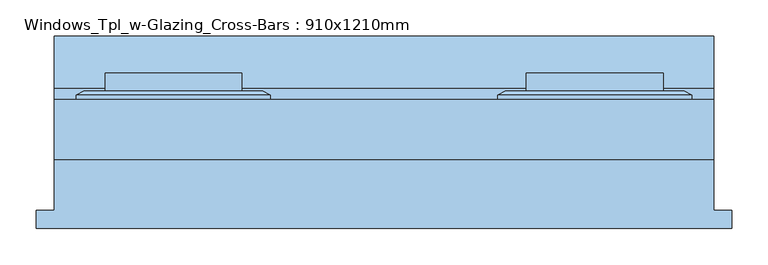
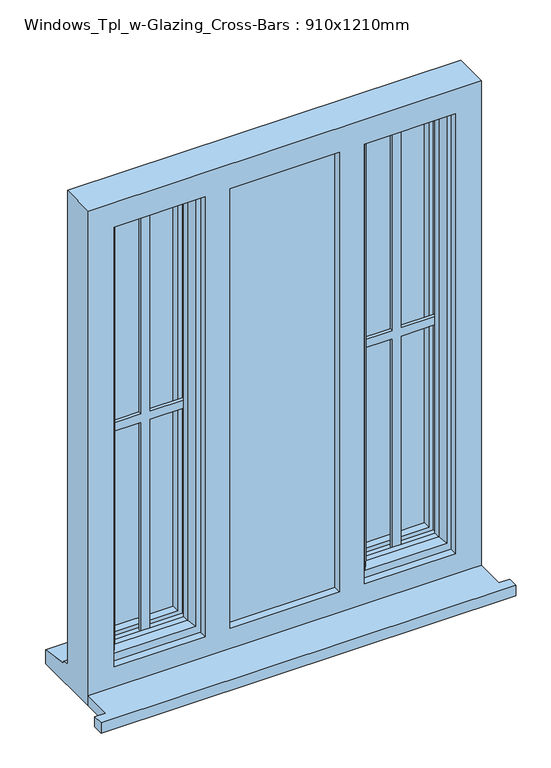
"""IFC4 building model written with IfcOpenShell, lengths in millimetres: window geometry, Windows_Tpl_w-Glazing_Cross-Bars : 910x1210mm."""

from ifc_helpers import new_model, si_unit, frame, origin, place, context, project, spatial, polyline, outline, extrude, faceted_brep, source, transform, mapped, element, save


def windows_tpl_w_glazing_cross_bars_910x1210mm_e0b59135(model_context):
    return source(origin(), model_context, "Body", "SolidModel", [
        extrude(outline(polyline([(-906.6666667, -118.1434322), (-906.6666667, -93.1434322), (-881.6666667, -93.1434322), (-881.6666667, -22.9434322), (28.3333333, -22.9434322), (28.3333333, -93.1434322), (53.3333333, -93.1434322), (53.3333333, -118.1434322), (-906.6666667, -118.1434322)])), frame((0.0, 0.0, 900.0), z_axis=(0.0, 0.0, 1.0), x_axis=(1.0, 0.0, 0.0)), (0.0, 0.0, 1.0), 25.0),
        faceted_brep([(-270.0, 60.0565678, 2080.0), (-270.0, 65.8300705, 2080.0), (-270.0, 65.8300705, 953.0), (-270.0, 60.0565678, 953.0), (-260.0, -4.9434322, 2070.0), (-260.0, 60.0565678, 2070.0), (-260.0, 60.0565678, 963.0), (-260.0, -4.9434322, 963.0), (-220.0, 9.5494677, 2030.0), (-230.1480377, -4.9434322, 2040.1480377), (-230.1480377, -4.9434322, 992.8519623), (-220.0, 9.5494677, 1003.0), (-220.0, 24.0565678, 2030.0), (-220.0, 24.0565678, 1003.0), (-230.0, 48.0565678, 2040.0), (-230.0, 24.0565678, 2040.0), (-230.0, 24.0565678, 993.0), (-230.0, 48.0565678, 993.0), (-220.0, 65.8300705, 2030.0), (-220.0, 48.0565678, 2030.0), (-220.0, 48.0565678, 1003.0), (-220.0, 65.8300705, 1003.0), (-237.4457548, 71.6035732, 2047.4457548), (-237.4457548, 71.6035732, 985.5542452), (-259.2153903, 71.6035732, 2069.2153903), (-259.2153903, 71.6035732, 963.7846097), (-1.6666667, 65.8300705, 953.0), (-1.6666667, 60.0565678, 953.0), (-11.6666667, 60.0565678, 963.0), (-11.6666667, -4.9434322, 963.0), (-41.5186289, -4.9434322, 992.8519623), (-51.6666667, 9.5494677, 1003.0), (-51.6666667, 24.0565678, 1003.0), (-41.6666667, 24.0565678, 993.0), (-41.6666667, 48.0565678, 993.0), (-51.6666667, 48.0565678, 1003.0), (-51.6666667, 65.8300705, 1003.0), (-34.2209119, 71.6035732, 985.5542452), (-12.4512764, 71.6035732, 963.7846097), (-1.6666667, 65.8300705, 2080.0), (-1.6666667, 60.0565678, 2080.0), (-11.6666667, 60.0565678, 2070.0), (-11.6666667, -4.9434322, 2070.0), (-41.5186289, -4.9434322, 2040.1480377), (-51.6666667, 9.5494677, 2030.0), (-51.6666667, 24.0565678, 2030.0), (-41.6666667, 24.0565678, 2040.0), (-41.6666667, 48.0565678, 2040.0), (-51.6666667, 48.0565678, 2030.0), (-51.6666667, 65.8300705, 2030.0), (-34.2209119, 71.6035732, 2047.4457548), (-12.4512764, 71.6035732, 2069.2153903)], [[[0, 1, 2, 3]], [[4, 5, 6, 7]], [[8, 9, 10, 11]], [[12, 8, 11, 13]], [[14, 15, 16, 17]], [[18, 19, 20, 21]], [[22, 18, 21, 23]], [[1, 24, 25, 2]], [[3, 2, 26, 27]], [[7, 6, 28, 29]], [[11, 10, 30, 31]], [[13, 11, 31, 32]], [[17, 16, 33, 34]], [[21, 20, 35, 36]], [[23, 21, 36, 37]], [[2, 25, 38, 26]], [[27, 26, 39, 40]], [[29, 28, 41, 42]], [[31, 30, 43, 44]], [[32, 31, 44, 45]], [[34, 33, 46, 47]], [[36, 35, 48, 49]], [[37, 36, 49, 50]], [[26, 38, 51, 39]], [[40, 39, 1, 0]], [[3, 27, 40, 0], [5, 41, 28, 6]], [[42, 41, 5, 4]], [[7, 29, 42, 4], [9, 43, 30, 10]], [[44, 43, 9, 8]], [[45, 44, 8, 12]], [[15, 46, 33, 16], [13, 32, 45, 12]], [[47, 46, 15, 14]], [[17, 34, 47, 14], [19, 48, 35, 20]], [[49, 48, 19, 18]], [[50, 49, 18, 22]], [[24, 51, 38, 25], [23, 37, 50, 22]], [[39, 51, 24, 1]]]),
        faceted_brep([(-583.3333333, 60.0565678, 2080.0), (-583.3333333, 65.8300705, 2080.0), (-851.6666667, 65.8300705, 2080.0), (-851.6666667, 60.0565678, 2080.0), (-593.3333333, -4.9434322, 2070.0), (-593.3333333, 60.0565678, 2070.0), (-841.6666667, 60.0565678, 2070.0), (-841.6666667, -4.9434322, 2070.0), (-633.3333333, 9.5494677, 2030.0), (-623.1852956, -4.9434322, 2040.1480377), (-811.8147044, -4.9434322, 2040.1480377), (-801.6666667, 9.5494677, 2030.0), (-633.3333333, 24.0565678, 2030.0), (-801.6666667, 24.0565678, 2030.0), (-623.3333333, 48.0565678, 2040.0), (-623.3333333, 24.0565678, 2040.0), (-811.6666667, 24.0565678, 2040.0), (-811.6666667, 48.0565678, 2040.0), (-633.3333333, 65.8300705, 2030.0), (-633.3333333, 48.0565678, 2030.0), (-801.6666667, 48.0565678, 2030.0), (-801.6666667, 65.8300705, 2030.0), (-615.8875785, 71.6035732, 2047.4457548), (-819.1124215, 71.6035732, 2047.4457548), (-594.117943, 71.6035732, 2069.2153903), (-840.882057, 71.6035732, 2069.2153903), (-851.6666667, 65.8300705, 953.0), (-851.6666667, 60.0565678, 953.0), (-841.6666667, 60.0565678, 963.0), (-841.6666667, -4.9434322, 963.0), (-811.8147044, -4.9434322, 992.8519623), (-801.6666667, 9.5494677, 1003.0), (-801.6666667, 24.0565678, 1003.0), (-811.6666667, 24.0565678, 993.0), (-811.6666667, 48.0565678, 993.0), (-801.6666667, 48.0565678, 1003.0), (-801.6666667, 65.8300705, 1003.0), (-819.1124215, 71.6035732, 985.5542452), (-840.882057, 71.6035732, 963.7846097), (-583.3333333, 65.8300705, 953.0), (-583.3333333, 60.0565678, 953.0), (-593.3333333, 60.0565678, 963.0), (-593.3333333, -4.9434322, 963.0), (-623.1852956, -4.9434322, 992.8519623), (-633.3333333, 9.5494677, 1003.0), (-633.3333333, 24.0565678, 1003.0), (-623.3333333, 24.0565678, 993.0), (-623.3333333, 48.0565678, 993.0), (-633.3333333, 48.0565678, 1003.0), (-633.3333333, 65.8300705, 1003.0), (-615.8875785, 71.6035732, 985.5542452), (-594.117943, 71.6035732, 963.7846097)], [[[0, 1, 2, 3]], [[4, 5, 6, 7]], [[8, 9, 10, 11]], [[12, 8, 11, 13]], [[14, 15, 16, 17]], [[18, 19, 20, 21]], [[22, 18, 21, 23]], [[1, 24, 25, 2]], [[3, 2, 26, 27]], [[7, 6, 28, 29]], [[11, 10, 30, 31]], [[13, 11, 31, 32]], [[17, 16, 33, 34]], [[21, 20, 35, 36]], [[23, 21, 36, 37]], [[2, 25, 38, 26]], [[27, 26, 39, 40]], [[0, 3, 27, 40], [41, 28, 6, 5]], [[29, 28, 41, 42]], [[4, 7, 29, 42], [43, 30, 10, 9]], [[31, 30, 43, 44]], [[32, 31, 44, 45]], [[46, 33, 16, 15], [12, 13, 32, 45]], [[34, 33, 46, 47]], [[14, 17, 34, 47], [48, 35, 20, 19]], [[36, 35, 48, 49]], [[37, 36, 49, 50]], [[51, 38, 25, 24], [22, 23, 37, 50]], [[26, 38, 51, 39]], [[40, 39, 1, 0]], [[42, 41, 5, 4]], [[44, 43, 9, 8]], [[45, 44, 8, 12]], [[47, 46, 15, 14]], [[49, 48, 19, 18]], [[50, 49, 18, 22]], [[39, 51, 24, 1]]]),
        extrude(outline(polyline([(993.0, -145.8333333), (993.0, -125.8333333), (1506.5, -125.8333333), (1506.5, -41.6666667), (1526.5, -41.6666667), (1526.5, -125.8333333), (2040.1480377, -125.8333333), (2040.1480377, -145.8333333), (1526.5, -145.8333333), (1526.5, -230.1480377), (1506.5, -230.1480377), (1506.5, -145.8333333), (993.0, -145.8333333)])), frame((0.0, 32.0565678, 0.0), z_axis=(0.0, 1.0, 0.0), x_axis=(0.0, 0.0, 1.0)), (0.0, 0.0, 1.0), 8.0),
        extrude(outline(polyline([(993.0, -727.5), (993.0, -707.5), (1506.5, -707.5), (1506.5, -623.3333333), (1526.5, -623.3333333), (1526.5, -707.5), (2040.1480377, -707.5), (2040.1480377, -727.5), (1526.5, -727.5), (1526.5, -811.6666667), (1506.5, -811.6666667), (1506.5, -727.5), (993.0, -727.5)])), frame((0.0, 32.0565678, 0.0), z_axis=(0.0, 1.0, 0.0), x_axis=(0.0, 0.0, 1.0)), (0.0, 0.0, 1.0), 8.0),
        extrude(outline(polyline([(963.0, -436.6666667), (963.0, -416.6666667), (1506.5, -416.6666667), (1506.5, -290.0), (1526.5, -290.0), (1526.5, -416.6666667), (2070.0, -416.6666667), (2070.0, -436.6666667), (1526.5, -436.6666667), (1526.5, -563.3333333), (1506.5, -563.3333333), (1506.5, -436.6666667), (963.0, -436.6666667)])), frame((0.0, 3.0565678, 0.0), z_axis=(0.0, 1.0, 0.0), x_axis=(0.0, 0.0, 1.0)), (0.0, 0.0, 1.0), 8.0),
        faceted_brep([(28.3333333, -22.9434322, 2110.0), (-881.6666667, -22.9434322, 2110.0), (-881.6666667, -22.9434322, 900.0), (28.3333333, -22.9434322, 900.0), (-31.6666667, -22.9434322, 2050.0), (-31.6666667, -22.9434322, 975.0), (-242.0, -22.9434322, 975.0), (-242.0, -22.9434322, 2050.0), (-300.0, -22.9434322, 2050.0), (-300.0, -22.9434322, 975.0), (-553.3333333, -22.9434322, 975.0), (-553.3333333, -22.9434322, 2050.0), (-611.3333333, -22.9434322, 2050.0), (-611.3333333, -22.9434322, 975.0), (-821.6666667, -22.9434322, 975.0), (-821.6666667, -22.9434322, 2050.0), (-881.6666667, 60.0565678, 2110.0), (-881.6666667, 60.0565678, 951.0), (-881.6666667, 75.0565678, 949.68767), (-881.6666667, 75.0565678, 944.7449676), (-881.6666667, 147.5565678, 933.8088847), (-881.6666667, 147.5565678, 900.0), (28.3333333, 60.0565678, 2110.0), (28.3333333, 60.0565678, 951.0), (-841.6666667, 60.0565678, 2070.0), (-841.6666667, 60.0565678, 963.0), (-593.3333333, 60.0565678, 963.0), (-593.3333333, 60.0565678, 2070.0), (-553.3333333, 60.0565678, 2070.0), (-553.3333333, 60.0565678, 963.0), (-300.0, 60.0565678, 963.0), (-300.0, 60.0565678, 2070.0), (-260.0, 60.0565678, 2070.0), (-260.0, 60.0565678, 963.0), (-11.6666667, 60.0565678, 963.0), (-11.6666667, 60.0565678, 2070.0), (-841.6666667, -4.9434322, 2070.0), (-841.6666667, -4.9434322, 963.0), (-563.3333333, -4.9434322, 2070.0), (-290.0, -4.9434322, 2070.0), (-290.0, -4.9434322, 963.0), (-563.3333333, -4.9434322, 963.0), (-300.0, -4.9434322, 2050.0), (-553.3333333, -4.9434322, 2050.0), (-553.3333333, -4.9434322, 975.0), (-300.0, -4.9434322, 975.0), (-260.0, -4.9434322, 2070.0), (-11.6666667, -4.9434322, 2070.0), (-11.6666667, -4.9434322, 963.0), (-260.0, -4.9434322, 963.0), (-31.6666667, -4.9434322, 2050.0), (-242.0, -4.9434322, 2050.0), (-242.0, -4.9434322, 975.0), (-31.6666667, -4.9434322, 975.0), (-593.3333333, -4.9434322, 2070.0), (-593.3333333, -4.9434322, 963.0), (-611.3333333, -4.9434322, 2050.0), (-821.6666667, -4.9434322, 2050.0), (-821.6666667, -4.9434322, 975.0), (-611.3333333, -4.9434322, 975.0), (-553.3333333, 19.0565678, 2070.0), (-300.0, 19.0565678, 2070.0), (-290.0, 19.0565678, 2070.0), (-563.3333333, 19.0565678, 2070.0), (28.3333333, 147.5565678, 900.0), (28.3333333, 147.5565678, 933.8088847), (28.3333333, 75.0565678, 944.7449676), (28.3333333, 75.0565678, 949.68767), (-553.3333333, 19.0565678, 963.0), (-563.3333333, 19.0565678, 963.0), (-290.0, 19.0565678, 963.0), (-300.0, 19.0565678, 963.0)], [[[0, 1, 2, 3], [4, 5, 6, 7], [8, 9, 10, 11], [12, 13, 14, 15]], [[2, 1, 16, 17, 18, 19, 20, 21]], [[17, 16, 22, 23], [24, 25, 26, 27], [28, 29, 30, 31], [32, 33, 34, 35]], [[25, 24, 36, 37]], [[38, 39, 40, 41], [42, 43, 44, 45]], [[46, 47, 48, 49], [50, 51, 52, 53]], [[36, 54, 55, 37], [56, 57, 58, 59]], [[57, 15, 14, 58]], [[1, 0, 22, 16]], [[36, 24, 27, 54]], [[35, 47, 46, 32]], [[60, 28, 31, 61, 62, 39, 38, 63]], [[15, 57, 56, 12]], [[50, 4, 7, 51]], [[11, 43, 42, 8]], [[23, 22, 0, 3, 64, 65, 66, 67]], [[35, 34, 48, 47]], [[4, 50, 53, 5]], [[43, 11, 10, 44]], [[12, 56, 59, 13]], [[27, 26, 55, 54]], [[29, 28, 60, 68]], [[68, 60, 63, 69]], [[69, 63, 38, 41]], [[62, 70, 40, 39]], [[70, 62, 61, 71]], [[71, 61, 31, 30]], [[33, 32, 46, 49]], [[51, 7, 6, 52]], [[8, 42, 45, 9]], [[64, 3, 2, 21]], [[65, 64, 21, 20]], [[66, 65, 20, 19]], [[67, 66, 19, 18]], [[23, 67, 18, 17]], [[26, 25, 37, 55]], [[34, 33, 49, 48]], [[41, 40, 70, 71, 30, 29, 68, 69]], [[6, 5, 53, 52]], [[45, 44, 10, 9]], [[59, 58, 14, 13]]]),
        extrude(outline(polyline([(-563.3333333, 19.0565678), (-290.0, 19.0565678), (-290.0, -4.9434322), (-563.3333333, -4.9434322), (-563.3333333, 19.0565678)])), frame((0.0, 0.0, 963.0), z_axis=(0.0, 0.0, 1.0), x_axis=(1.0, 0.0, 0.0)), (0.0, 0.0, 1.0), 1107.0),
        extrude(outline(polyline([(-623.3333333, 72.4565678), (-811.6666667, 72.4565678), (-811.6666667, 96.4565678), (-623.3333333, 96.4565678), (-623.3333333, 72.4565678)])), frame((0.0, 0.0, 993.0), z_axis=(0.0, 0.0, 1.0), x_axis=(1.0, 0.0, 0.0)), (0.0, 0.0, 1.0), 1047.0),
        extrude(outline(polyline([(-41.5186289, 72.4565678), (-230.1480377, 72.4565678), (-230.1480377, 96.4565678), (-41.5186289, 96.4565678), (-41.5186289, 72.4565678)])), frame((0.0, 0.0, 992.8519623), z_axis=(0.0, 0.0, 1.0), x_axis=(1.0, 0.0, 0.0)), (0.0, 0.0, 1.0), 1047.2960754),
    ])


if __name__ == "__main__":
    model = new_model("IFC4")
    model_context = context("Model", 3, world=origin())
    ifc_project = project(units=[si_unit("LENGTHUNIT", "METRE", prefix="MILLI")], contexts=[model_context])
    site = spatial("IfcSite", under=ifc_project)
    building = spatial("IfcBuilding", under=site)
    placement = place(None, origin())
    windows_tpl_w_glazing_cross_bars_910x1210mm_shape = windows_tpl_w_glazing_cross_bars_910x1210mm_e0b59135(model_context)
    element("IfcWindow", 1, ObjectType="Windows_Tpl_w-Glazing_Cross-Bars : 910x1210mm", at=placement, inside=building, context=model_context, shape_type="MappedRepresentation", body=[
        mapped(windows_tpl_w_glazing_cross_bars_910x1210mm_shape, transform((0.0, 0.0, 0.0), x_axis=(1.0, 0.0, 0.0), y_axis=(0.0, 1.0, 0.0), z_axis=(0.0, 0.0, 1.0))),
    ])
    save(model, "model.ifc")

# Revit data of these elements
# Type "Windows_Tpl_w-Glazing_Cross-Bars : 910x1210mm"
#   Type Mark = "25"
#   Operation = "TriplePanelVertical"
#   Construction Type Id = "GSP4R"
#   Manufacturer = "Revit"
#   Keynote = "L10"
#   Analytic Construction = "1/8 in Pilkington single glazing"
#   Wrap Layers (Ext) from Ext = 0' - 4.03543"
#   Wrap Layers (Int) from Ext = 0' - 6.98819"
#   Window Board Projection = 0' - 0.98425"
#   Window Board Extension = 0' - 0.98425"
#   Visual Light Transmittance = 0.9
#   Solar Heat Gain Coefficient = 0.78
#   Rough Width = 2' - 11.82677"
#   Rough Height = 3' - 11.6378"
#   Height = 3' - 11.6378"
#   Width = 2' - 11.82677"
#   Heat Transfer Coefficient (U) = 0.6496 BTU/(h·ft²·°F)
#   Glazing Thickness = 0' - 0.94488"
#   Glazing Bar Thickness = 0' - 0.7874"
#   FrameOffset - External = 0' - 1.9685"
#   Frame Depth = 0' - 2.55906"
#   Default Head Height = 6' - 11.07087"
#   Cill Depth = 0' - 3.44488"
#   Cavity Closer Width = 0' - 1.9685"
#   Cavity Closer Offset from Ext = 0' - 4.03543"
#   Cavity Closer Depth = 0' - 3.34646"
#   Vis - Glazing Bars = yes
#   Vis - Cavity Closers = yes
#   Define Thermal Properties by = 1
#   Material Trim = Window Frame
#   Material Glazing Bars = Window Frame
#   Material Glass = Glass
#   Material Frame = Window Frame
#   Wall Closure = (empty or 0)
# Element 1 (IfcWindow, "Windows_Tpl_w-Glazing_Cross-Bars : 910x1210mm")
#   Materials on its faces: "Window Frame", "Glass"
# Materials
#   "Window Frame": colour RGB 249 249 249, transparency 0
#   "Glass": class "Glass", colour RGB 0 128 192, transparency 0.75, Description = "Soda Lime Glass", Cost = 0
